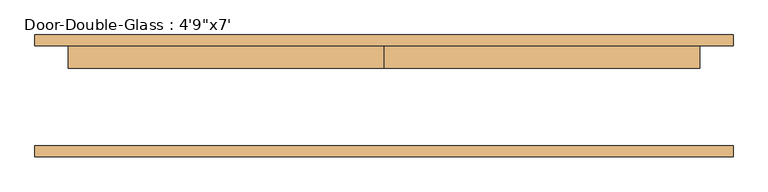
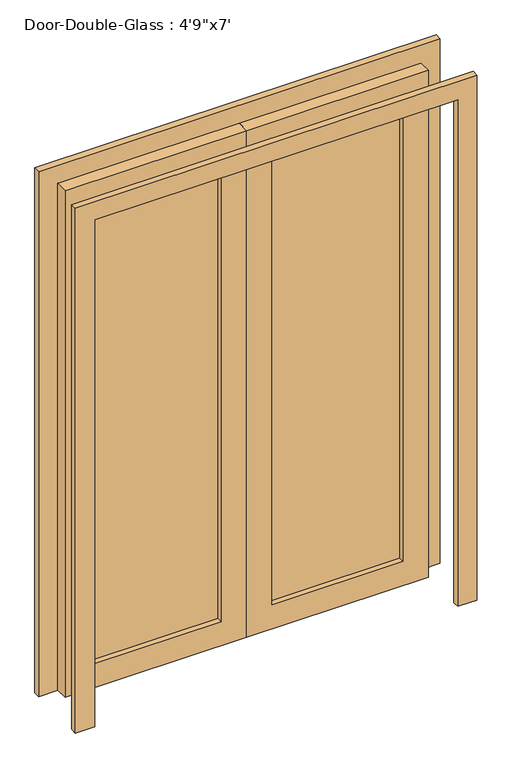
"""IFC4 building model written with IfcOpenShell, lengths in millimetres: door geometry."""

from ifc_helpers import new_model, si_unit, frame, origin, place, context, project, spatial, polyline, outline, extrude, source, transform, mapped, element, save


def door_7b3e5dee(model_context):
    return source(origin(), model_context, "Body", "SweptSolid", [
        extrude(outline(polyline([(2133.6, 723.9), (2133.6, 0.0), (0.0, 0.0), (0.0, 723.9), (2133.6, 723.9)]), holes=[polyline([(2032.0, 622.3), (101.6, 622.3), (101.6, 101.6), (2032.0, 101.6), (2032.0, 622.3)])]), frame((0.0, 65.88125, 0.0), z_axis=(0.0, 1.0, 0.0), x_axis=(0.0, 0.0, 1.0)), (0.0, 0.0, 1.0), 50.8),
        extrude(outline(polyline([(2133.6, -723.9), (0.0, -723.9), (0.0, 0.0), (2133.6, 0.0), (2133.6, -723.9)]), holes=[polyline([(2032.0, -622.3), (2032.0, -101.6), (101.6, -101.6), (101.6, -622.3), (2032.0, -622.3)])]), frame((0.0, 65.88125, 0.0), z_axis=(0.0, 1.0, 0.0), x_axis=(0.0, 0.0, 1.0)), (0.0, 0.0, 1.0), 50.8),
        extrude(outline(polyline([(-622.3, 94.45625), (-101.6, 94.45625), (-101.6, 88.10625), (-622.3, 88.10625), (-622.3, 94.45625)])), frame((0.0, 0.0, 101.6), z_axis=(0.0, 0.0, 1.0), x_axis=(1.0, 0.0, 0.0)), (0.0, 0.0, 1.0), 1930.4),
        extrude(outline(polyline([(101.6, 94.45625), (622.3, 94.45625), (622.3, 88.10625), (101.6, 88.10625), (101.6, 94.45625)])), frame((0.0, 0.0, 101.6), z_axis=(0.0, 0.0, 1.0), x_axis=(1.0, 0.0, 0.0)), (0.0, 0.0, 1.0), 1930.4),
        extrude(outline(polyline([(0.0, 800.1), (2209.8, 800.1), (2209.8, -800.1), (0.0, -800.1), (0.0, -723.9), (2133.6, -723.9), (2133.6, 723.9), (0.0, 723.9), (0.0, 800.1)])), frame((0.0, -137.31875, 0.0), z_axis=(0.0, 1.0, 0.0), x_axis=(0.0, 0.0, 1.0)), (0.0, 0.0, 1.0), 25.4),
        extrude(outline(polyline([(0.0, 800.1), (2209.8, 800.1), (2209.8, -800.1), (0.0, -800.1), (0.0, -723.9), (2133.6, -723.9), (2133.6, 723.9), (0.0, 723.9), (0.0, 800.1)])), frame((0.0, 116.68125, 0.0), z_axis=(0.0, 1.0, 0.0), x_axis=(0.0, 0.0, 1.0)), (0.0, 0.0, 1.0), 25.4),
    ])


if __name__ == "__main__":
    model = new_model("IFC4")
    model_context = context("Model", 3, world=origin())
    ifc_project = project(units=[si_unit("LENGTHUNIT", "METRE", prefix="MILLI")], contexts=[model_context])
    site = spatial("IfcSite", under=ifc_project)
    building = spatial("IfcBuilding", under=site)
    placement = place(None, origin())
    door_shape = door_7b3e5dee(model_context)
    element("IfcDoor", 1, ObjectType="Door-Double-Glass : 4'9\"x7'", at=placement, inside=building, context=model_context, shape_type="MappedRepresentation", body=[
        mapped(door_shape, transform((0.0, 0.0, 0.0), x_axis=(1.0, 0.0, 0.0), y_axis=(0.0, 1.0, 0.0), z_axis=(0.0, 0.0, 1.0))),
    ])
    save(model, "model.ifc")

# Revit data of these elements
# Type "Door-Double-Glass : 4'9\"x7'"
#   Type Mark = "9"
#   Construction Type Id = "opn-d45"
#   Assembly Code = "C1020"
#   Analytic Construction = "Wood frame, double glass door "
#   W = 2' - 4 1/2"
#   Thickness = 0' - 2"
#   Thermal Resistance (R) = 1.8150 (h·ft²·°F)/BTU
#   Swing Angle [instance default] = 90.00°
#   Heat Transfer Coefficient (U) = 0.5510 BTU/(h·ft²·°F)
#   Height = 7' - 0"
#   Bottom Rail = 0' - 4"
#   Top Rail = 0' - 4"
#   Stiles = 0' - 4"
#   Trim Projection = 0' - 1"
#   Trim Width = 0' - 3"
#   Width = 4' - 9"
#   Define Thermal Properties by = 1
#   Glazing = Glass
#   Panel Material = Wood - Birch - Solid Stained Light Low Gloss
#   Trim Material = Paint - Sienna
#   Visual Light Transmittance = 0
#   Solar Heat Gain Coefficient = 0
#   Function = (empty or 0)
#   Wall Closure = (empty or 0)
# Element 1 (IfcDoor, "Door-Double-Glass : 4'9\"x7'")
#   Materials on its faces: "Wood - Birch - Solid Stained Light Low Gloss", "Paint - Sienna", "Glass"
# Materials
#   "Glass": class "Glass", colour RGB 154 182 205, transparency 0.85, Description = "Soda Lime Glass", Cost = 0
#   "Wood - Birch - Solid Stained Light Low Gloss": class "Wood", colour RGB 210 159 95, transparency 0, Cost = 0
#   "Paint - Sienna": colour RGB 118 70 51, transparency 0, Cost = 0
